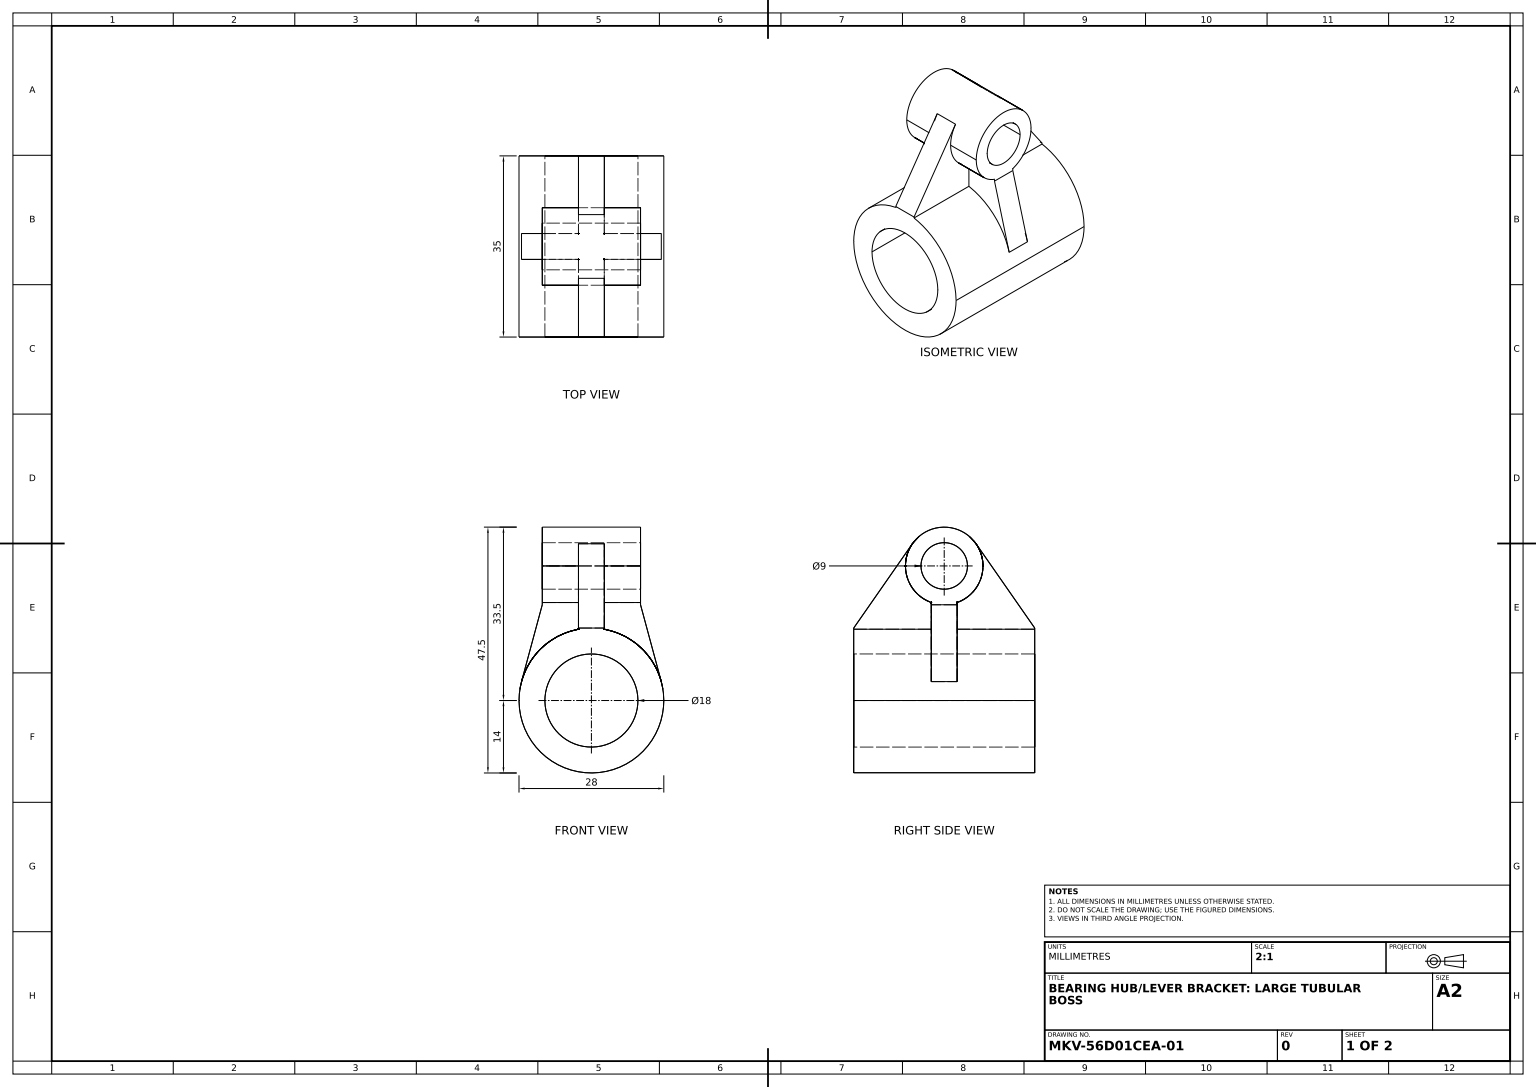
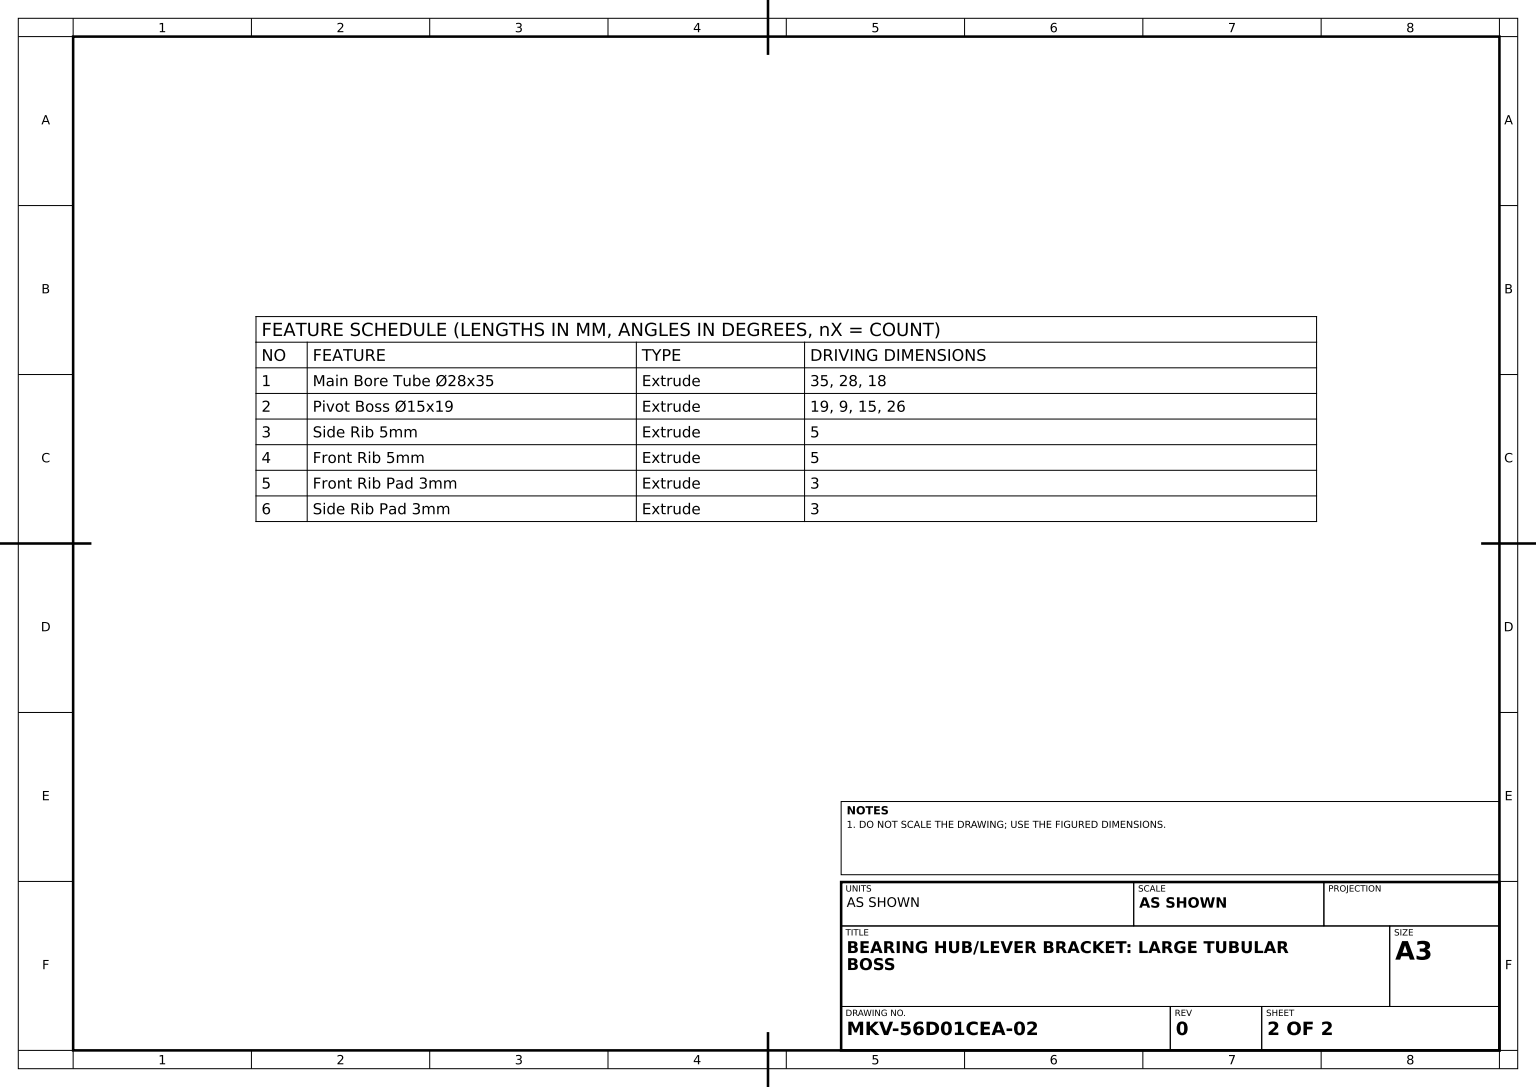
from build123d import *

# Parameters (mm, degrees)
MAIN_BORE_PROFILE_28_18_R   = 14
MAIN_BORE_PROFILE_28_18_R_2 = 9
MAIN_BORE_TUBE_28X35_DEPTH  = 17.5
PIVOT_BOSS_PROFILE_15_9_R   = 7.5
PIVOT_BOSS_PROFILE_15_9_R_2 = 4.5
PIVOT_BOSS_15X19_DEPTH      = 9.5
SIDE_RIB_5MM_DEPTH          = 2.5
FRONT_RIB_5MM_DEPTH         = 2.5
FRONT_RIB_PAD_PROFILE_W     = 19
FRONT_RIB_PAD_PROFILE_H     = 5
FRONT_RIB_PAD_3MM_DEPTH     = 3
SIDE_RIB_PAD_PROFILE_W      = 5
SIDE_RIB_PAD_PROFILE_H      = 35
SIDE_RIB_PAD_3MM_DEPTH      = 3


with BuildPart() as part:
    # Main Bore Profile Ø28-Ø18 → Main Bore Tube Ø28x35 (new, symmetric)
    with BuildSketch(Plane.XY):
        Circle(MAIN_BORE_PROFILE_28_18_R)
        Circle(MAIN_BORE_PROFILE_28_18_R_2, mode=Mode.SUBTRACT)
    extrude(amount=MAIN_BORE_TUBE_28X35_DEPTH, both=True)



with BuildPart() as body_2:
    # Pivot Boss Profile Ø15-Ø9 → Pivot Boss Ø15x19 (new, symmetric)
    with BuildSketch(Plane(origin=(0, 0, 0), x_dir=(0, 0, -1), z_dir=(1, 0, 0))):
        with Locations((0, 26)):
            Circle(PIVOT_BOSS_PROFILE_15_9_R)
        with Locations((0, 26)):
            Circle(PIVOT_BOSS_PROFILE_15_9_R_2, mode=Mode.SUBTRACT)
    extrude(amount=PIVOT_BOSS_15X19_DEPTH, both=True)

    # Side Rib Profile → Side Rib 5mm (add, symmetric)
    with BuildSketch(Plane(origin=(0, 0, 0), x_dir=(0, 0, -1), z_dir=(1, 0, 0))):
        with BuildLine():
            Line((-17.5, 14), (-6.153967777, 30.287036342))
            ThreePointArc((-6.153967777, 30.287036342), (0, 18.5), (6.153967777, 30.287036342))
            Line((6.153967777, 30.287036342), (17.5, 14))
            Line((17.5, 14), (-17.5, 14))
        make_face()
    extrude(amount=SIDE_RIB_5MM_DEPTH, both=True)



with BuildPart() as body_3:
    # Front Rib Profile → Front Rib 5mm (new, symmetric)
    with BuildSketch(Plane.XY):
        with BuildLine():
            Line((-13.514557534, 3.654686672), (-9.5, 18.5))
            Line((-9.5, 18.5), (9.5, 18.5))
            Line((9.5, 18.5), (13.514557534, 3.654686672))
            ThreePointArc((13.514557534, 3.654686672), (0, 14), (-13.514557534, 3.654686672))
        make_face()
    extrude(amount=FRONT_RIB_5MM_DEPTH, both=True)


with BuildPart() as body_2_1:
    add(body_2.part)

    add(body_3.part)  # Front Rib Pad 3mm merges body 3
    # Front Rib Pad Profile → Front Rib Pad 3mm (add)
    with BuildSketch(Plane(origin=(0, 18.5, 0), x_dir=(1, 0, 0), z_dir=(0, 1, 0))):
        Rectangle(FRONT_RIB_PAD_PROFILE_W, FRONT_RIB_PAD_PROFILE_H)
    extrude(amount=FRONT_RIB_PAD_3MM_DEPTH)


with BuildPart() as part_1:
    add(part.part)

    add(body_2_1.part)  # Side Rib Pad 3mm merges body 2
    # Side Rib Pad Profile → Side Rib Pad 3mm (add)
    with BuildSketch(Plane.XZ.offset(-14)):
        Rectangle(SIDE_RIB_PAD_PROFILE_W, SIDE_RIB_PAD_PROFILE_H)
    extrude(amount=SIDE_RIB_PAD_3MM_DEPTH)


solid = part_1.part
